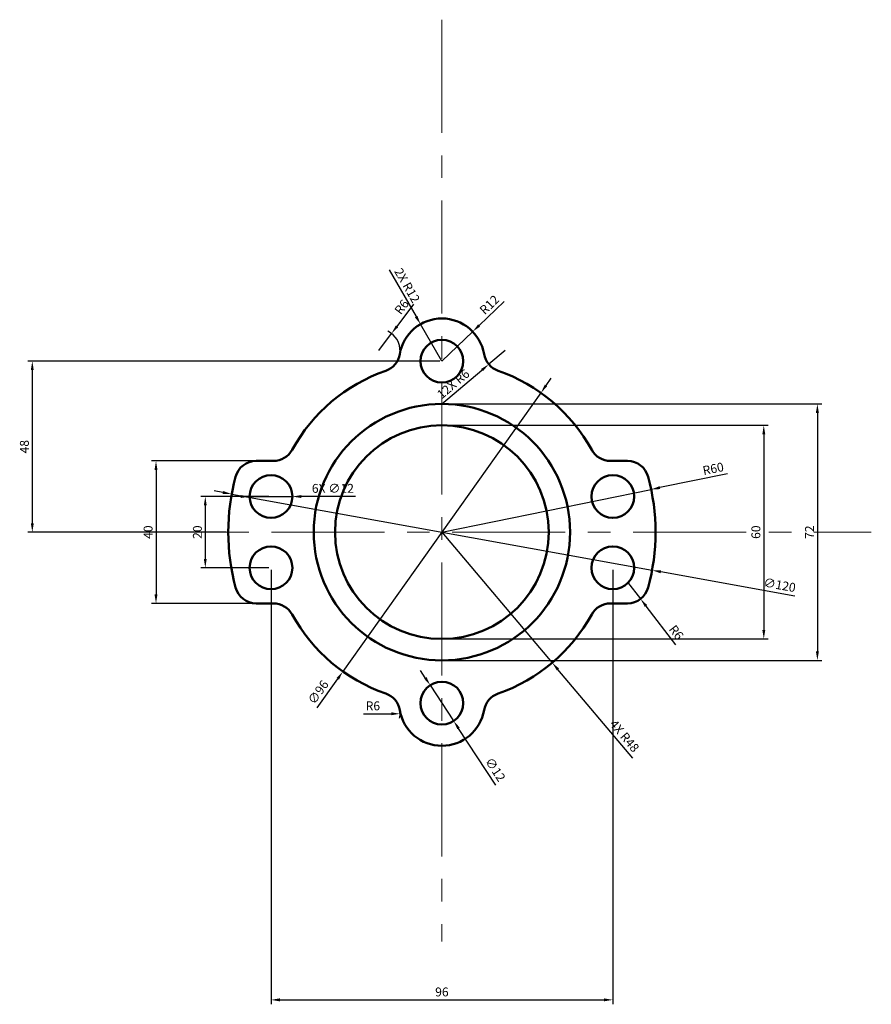
# Model space of a CAD drawing. Units: millimetres. Extents: x 2281 to 2520, y 1488 to 1764.
import ezdxf

# ---------------------------------------------------------------- set-up
doc = ezdxf.new("R2010")
doc.units = ezdxf.units.MM
doc.linetypes.add('CENTER', pattern=[50.8, 31.75, -6.35, 6.35, -6.35])
for name, color, linetype, lineweight in [('M-CNTR', 4, 'CENTER', 18), ('M-DIMS', 2, 'Continuous', 25), ('M-OUTL', 7, 'Continuous', 50)]:
    doc.layers.add(name, color=color, linetype=linetype, lineweight=lineweight)
doc.styles.get("Standard").update_dxf_attribs({"font": 'arial.ttf'})
doc.dimstyles.new('ISO-25', dxfattribs={"dimtxt": 2.5, "dimasz": 2.5, "dimexe": 1.25, "dimexo": 0.625, "dimtad": 1, "dimtxsty": 'Standard', "dimcen": 2.5, "dimadec": 0, "dimazin": 0, "dimtfac": 1, "dimtmove": 0, "dimatfit": 3, "dimfxl": 1, "dimarcsym": 0})

# ---------------------------------------------------------------- blocks, each defined once
blk = doc.blocks.new('*D1')
at = {"layer": 'Defpoints', "color": 0, "transparency": 16777216}
for p in [(2385.57, 1676.16), (2381.96, 1671.37)]:
    blk.add_point(p, dxfattribs=at)
at = {"layer": 'M-DIMS', "color": 0, "lineweight": -2, "transparency": 16777216}
for p, q in [((2391.76, 1684.37), (2387.08, 1678.16)), ((2381.96, 1671.37), (2385.57, 1676.16))]:
    blk.add_line(p, q, dxfattribs=at)
blk.add_arc((2381.96, 1671.37), 6, 356.3742, 64.8962, dxfattribs=at)
at = {"layer": 'M-DIMS', "color": 0, "transparency": 16777216}
blk.add_solid([(2386.75, 1678.41), (2387.41, 1677.91), (2385.57, 1676.16)], dxfattribs=at)
at = {"layer": 'M-DIMS', "color": 0, "transparency": 16777216, "insert": (2388.66, 1683.41), "char_height": 2.5, "attachment_point": 5, "rotation": 52.9596}
blk.add_mtext('R6', dxfattribs=at)
blk = doc.blocks.new('*D2')
at = {"layer": 'Defpoints', "color": 0, "transparency": 16777216}
for p in [(2408.36, 1676.69), (2399.71, 1668.37)]:
    blk.add_point(p, dxfattribs=at)
at = {"layer": 'M-DIMS', "color": 0, "lineweight": -2, "transparency": 16777216}
for p, q in [((2417.15, 1685.14), (2410.16, 1678.42)), ((2399.71, 1668.37), (2408.36, 1676.69))]:
    blk.add_line(p, q, dxfattribs=at)
at = {"layer": 'M-DIMS', "color": 0, "transparency": 16777216}
blk.add_solid([(2409.87, 1678.72), (2410.45, 1678.12), (2408.36, 1676.69)], dxfattribs=at)
at = {"layer": 'M-DIMS', "color": 0, "transparency": 16777216, "insert": (2413.26, 1684), "char_height": 2.5, "attachment_point": 5, "rotation": 43.8587}
blk.add_mtext('R12', dxfattribs=at)
blk = doc.blocks.new('*D3')
at = {"layer": 'Defpoints', "color": 0, "transparency": 16777216}
for p in [(2458.49, 1632.37), (2399.71, 1620.37)]:
    blk.add_point(p, dxfattribs=at)
at = {"layer": 'M-DIMS', "color": 0, "lineweight": -2, "transparency": 16777216}
for p, q in [((2479.89, 1636.74), (2460.94, 1632.87)), ((2399.71, 1620.37), (2458.49, 1632.37))]:
    blk.add_line(p, q, dxfattribs=at)
at = {"layer": 'M-DIMS', "color": 0, "transparency": 16777216}
blk.add_solid([(2460.86, 1633.28), (2461.03, 1632.46), (2458.49, 1632.37)], dxfattribs=at)
at = {"layer": 'M-DIMS', "color": 0, "transparency": 16777216, "insert": (2475.97, 1637.88), "char_height": 2.5, "attachment_point": 5, "rotation": 11.5363}
blk.add_mtext('R60', dxfattribs=at)
blk = doc.blocks.new('*D4')
at = {"layer": 'Defpoints', "color": 0, "transparency": 16777216}
for p in [(2451.86, 1606.37), (2455.51, 1601.61)]:
    blk.add_point(p, dxfattribs=at)
at = {"layer": 'M-DIMS', "color": 0, "lineweight": -2, "transparency": 16777216}
for p, q in [((2451.86, 1606.37), (2455.51, 1601.61)), ((2465.39, 1588.76), (2457.04, 1599.63))]:
    blk.add_line(p, q, dxfattribs=at)
at = {"layer": 'M-DIMS', "color": 0, "transparency": 16777216}
blk.add_solid([(2457.37, 1599.89), (2456.71, 1599.38), (2455.51, 1601.61)], dxfattribs=at)
at = {"layer": 'M-DIMS', "color": 0, "transparency": 16777216, "insert": (2465.29, 1592.02), "char_height": 2.5, "attachment_point": 5, "rotation": 307.5279}
blk.add_mtext('R6', dxfattribs=at)
blk = doc.blocks.new('*D5')
at = {"layer": 'Defpoints', "color": 0, "transparency": 16777216}
for p in [(2396.41, 1577.39), (2403, 1567.36)]:
    blk.add_point(p, dxfattribs=at)
at = {"layer": 'M-DIMS', "color": 0, "lineweight": -2, "transparency": 16777216}
for p, q in [((2395.03, 1579.47), (2393.66, 1581.56)), ((2396.41, 1577.39), (2403, 1567.36)), ((2414.87, 1549.32), (2404.38, 1565.27))]:
    blk.add_line(p, q, dxfattribs=at)
at = {"layer": 'M-DIMS', "color": 0, "transparency": 16777216}
for points in [[(2395.38, 1579.7), (2394.69, 1579.25), (2396.41, 1577.39)], [(2404.72, 1565.5), (2404.03, 1565.04), (2403, 1567.36)]]:
    blk.add_solid(points, dxfattribs=at)
at = {"layer": 'M-DIMS', "color": 0, "transparency": 16777216, "insert": (2414.45, 1553.55), "char_height": 2.5, "attachment_point": 5, "rotation": 303.334}
blk.add_mtext('∅12', dxfattribs=at)
blk = doc.blocks.new('*D6')
at = {"layer": 'Defpoints', "color": 0, "transparency": 16777216}
for p in [(2381.96, 1569.37), (2387.96, 1569.37)]:
    blk.add_point(p, dxfattribs=at)
at = {"layer": 'M-DIMS', "color": 0, "lineweight": -2, "transparency": 16777216}
blk.add_line((2377.68, 1569.37), (2385.46, 1569.37), dxfattribs=at)
blk.add_arc((2381.96, 1569.37), 6, 348.0634, 3.6258, dxfattribs=at)
at = {"layer": 'M-DIMS', "color": 0, "transparency": 16777216}
blk.add_solid([(2385.46, 1569.79), (2385.46, 1568.96), (2387.96, 1569.37)], dxfattribs=at)
at = {"layer": 'M-DIMS', "color": 0, "transparency": 16777216, "insert": (2380.32, 1571.27), "char_height": 2.5, "attachment_point": 5}
blk.add_mtext('R6', dxfattribs=at)
blk = doc.blocks.new('*D7')
at = {"layer": 'Defpoints', "color": 0, "transparency": 16777216}
for p in [(2427.51, 1659.5), (2371.9, 1581.24)]:
    blk.add_point(p, dxfattribs=at)
at = {"layer": 'M-DIMS', "color": 0, "lineweight": -2, "transparency": 16777216}
for p, q in [((2428.95, 1661.54), (2430.4, 1663.58)), ((2427.51, 1659.5), (2371.9, 1581.24)), ((2364.64, 1571.01), (2370.46, 1579.21))]:
    blk.add_line(p, q, dxfattribs=at)
at = {"layer": 'M-DIMS', "color": 0, "transparency": 16777216}
for points in [[(2428.62, 1661.78), (2429.29, 1661.3), (2427.51, 1659.5)], [(2370.12, 1579.45), (2370.8, 1578.96), (2371.9, 1581.24)]]:
    blk.add_solid(points, dxfattribs=at)
at = {"layer": 'M-DIMS', "color": 0, "transparency": 16777216, "insert": (2365.22, 1575.23), "char_height": 2.5, "attachment_point": 5, "rotation": 54.6066}
blk.add_mtext('∅96', dxfattribs=at)
blk = doc.blocks.new('*D8')
at = {"layer": 'Defpoints', "color": 0, "transparency": 16777216}
for p in [(2351.71, 1630.37), (2333.25, 1610.37), (2351.71, 1610.37)]:
    blk.add_point(p, dxfattribs=at)
at = {"layer": 'M-DIMS', "color": 0, "lineweight": -2, "transparency": 16777216}
for p, q in [((2351.08, 1630.37), (2332, 1630.37)), ((2333.25, 1627.87), (2333.25, 1612.87)), ((2351.08, 1610.37), (2332, 1610.37))]:
    blk.add_line(p, q, dxfattribs=at)
at = {"layer": 'M-DIMS', "color": 0, "transparency": 16777216}
for points in [[(2332.83, 1627.87), (2333.66, 1627.87), (2333.25, 1630.37)], [(2332.83, 1612.87), (2333.66, 1612.87), (2333.25, 1610.37)]]:
    blk.add_solid(points, dxfattribs=at)
at = {"layer": 'M-DIMS', "color": 0, "transparency": 16777216, "insert": (2331.35, 1620.37), "char_height": 2.5, "attachment_point": 5, "rotation": 90}
blk.add_mtext('20', dxfattribs=at)
blk = doc.blocks.new('*D9')
at = {"layer": 'Defpoints', "color": 0, "transparency": 16777216}
for p in [(2352.38, 1640.37), (2319.41, 1600.37), (2352.38, 1600.37)]:
    blk.add_point(p, dxfattribs=at)
at = {"layer": 'M-DIMS', "color": 0, "lineweight": -2, "transparency": 16777216}
for p, q in [((2351.75, 1640.37), (2318.16, 1640.37)), ((2319.41, 1637.87), (2319.41, 1602.87)), ((2351.75, 1600.37), (2318.16, 1600.37))]:
    blk.add_line(p, q, dxfattribs=at)
at = {"layer": 'M-DIMS', "color": 0, "transparency": 16777216}
for points in [[(2318.99, 1637.87), (2319.82, 1637.87), (2319.41, 1640.37)], [(2318.99, 1602.87), (2319.82, 1602.87), (2319.41, 1600.37)]]:
    blk.add_solid(points, dxfattribs=at)
at = {"layer": 'M-DIMS', "color": 0, "transparency": 16777216, "insert": (2317.51, 1620.37), "char_height": 2.5, "attachment_point": 5, "rotation": 90}
blk.add_mtext('40', dxfattribs=at)
blk = doc.blocks.new('*D10')
at = {"layer": 'Defpoints', "color": 0, "transparency": 16777216}
for p in [(2399.71, 1650.37), (2399.71, 1590.37), (2490.12, 1590.37)]:
    blk.add_point(p, dxfattribs=at)
at = {"layer": 'M-DIMS', "color": 0, "lineweight": -2, "transparency": 16777216}
for p, q in [((2400.33, 1650.37), (2491.37, 1650.37)), ((2490.12, 1647.87), (2490.12, 1592.87)), ((2400.33, 1590.37), (2491.37, 1590.37))]:
    blk.add_line(p, q, dxfattribs=at)
at = {"layer": 'M-DIMS', "color": 0, "transparency": 16777216}
for points in [[(2489.71, 1647.87), (2490.54, 1647.87), (2490.12, 1650.37)], [(2489.71, 1592.87), (2490.54, 1592.87), (2490.12, 1590.37)]]:
    blk.add_solid(points, dxfattribs=at)
at = {"layer": 'M-DIMS', "color": 0, "transparency": 16777216, "insert": (2488.22, 1620.37), "char_height": 2.5, "attachment_point": 5, "rotation": 90}
blk.add_mtext('60', dxfattribs=at)
blk = doc.blocks.new('*D11')
at = {"layer": 'Defpoints', "color": 0, "transparency": 16777216}
for p in [(2399.71, 1656.37), (2399.71, 1584.37), (2505.17, 1584.37)]:
    blk.add_point(p, dxfattribs=at)
at = {"layer": 'M-DIMS', "color": 0, "lineweight": -2, "transparency": 16777216}
for p, q in [((2400.33, 1656.37), (2506.42, 1656.37)), ((2505.17, 1653.87), (2505.17, 1586.87)), ((2400.33, 1584.37), (2506.42, 1584.37))]:
    blk.add_line(p, q, dxfattribs=at)
at = {"layer": 'M-DIMS', "color": 0, "transparency": 16777216}
for points in [[(2504.75, 1653.87), (2505.59, 1653.87), (2505.17, 1656.37)], [(2504.75, 1586.87), (2505.59, 1586.87), (2505.17, 1584.37)]]:
    blk.add_solid(points, dxfattribs=at)
at = {"layer": 'M-DIMS', "color": 0, "transparency": 16777216, "insert": (2503.29, 1620.37), "char_height": 2.5, "attachment_point": 5, "rotation": 90}
blk.add_mtext('72', dxfattribs=at)
blk = doc.blocks.new('BOLT-HOLE-D12')
blk.add_circle((6, 6), 6)
blk = doc.blocks.new('*D13')
at = {"layer": 'Defpoints', "color": 0, "transparency": 16777216}
for p in [(2351.71, 1610.37), (2447.71, 1610.37), (2447.71, 1489.03)]:
    blk.add_point(p, dxfattribs=at)
at = {"layer": 'M-DIMS', "color": 0, "lineweight": -2, "transparency": 16777216}
for p, q in [((2351.71, 1609.75), (2351.71, 1487.78)), ((2447.71, 1609.75), (2447.71, 1487.78)), ((2354.21, 1489.03), (2445.21, 1489.03))]:
    blk.add_line(p, q, dxfattribs=at)
at = {"layer": 'M-DIMS', "color": 0, "transparency": 16777216}
for points in [[(2354.21, 1489.45), (2354.21, 1488.61), (2351.71, 1489.03)], [(2445.21, 1489.45), (2445.21, 1488.61), (2447.71, 1489.03)]]:
    blk.add_solid(points, dxfattribs=at)
at = {"layer": 'M-DIMS', "color": 0, "transparency": 16777216, "insert": (2399.71, 1490.93), "char_height": 2.5, "attachment_point": 5}
blk.add_mtext('96', dxfattribs=at)
blk = doc.blocks.new('*D14')
at = {"layer": 'Defpoints', "color": 0, "transparency": 16777216}
for p in [(2399.71, 1668.37), (2284.66, 1620.37), (2339.71, 1620.37)]:
    blk.add_point(p, dxfattribs=at)
at = {"layer": 'M-DIMS', "color": 0, "lineweight": -2, "transparency": 16777216}
for p, q in [((2399.08, 1668.37), (2283.41, 1668.37)), ((2284.66, 1665.87), (2284.66, 1622.87)), ((2339.08, 1620.37), (2283.41, 1620.37))]:
    blk.add_line(p, q, dxfattribs=at)
at = {"layer": 'M-DIMS', "color": 0, "transparency": 16777216}
for points in [[(2284.24, 1665.87), (2285.07, 1665.87), (2284.66, 1668.37)], [(2284.24, 1622.87), (2285.07, 1622.87), (2284.66, 1620.37)]]:
    blk.add_solid(points, dxfattribs=at)
at = {"layer": 'M-DIMS', "color": 0, "transparency": 16777216, "insert": (2282.76, 1644.37), "char_height": 2.5, "attachment_point": 5, "rotation": 90}
blk.add_mtext('48', dxfattribs=at)
blk = doc.blocks.new('*D15')
at = {"layer": 'Defpoints', "color": 0, "transparency": 16777216}
for p in [(2340.67, 1631.06), (2458.75, 1609.69)]:
    blk.add_point(p, dxfattribs=at)
at = {"layer": 'M-DIMS', "color": 0, "lineweight": -2, "transparency": 16777216}
for p, q in [((2338.21, 1631.51), (2335.75, 1631.95)), ((2340.67, 1631.06), (2458.75, 1609.69)), ((2498.84, 1602.43), (2461.21, 1609.24))]:
    blk.add_line(p, q, dxfattribs=at)
at = {"layer": 'M-DIMS', "color": 0, "transparency": 16777216}
for points in [[(2338.28, 1631.92), (2338.13, 1631.1), (2340.67, 1631.06)], [(2461.28, 1609.65), (2461.13, 1608.83), (2458.75, 1609.69)]]:
    blk.add_solid(points, dxfattribs=at)
at = {"layer": 'M-DIMS', "color": 0, "transparency": 16777216, "insert": (2494.52, 1605.21), "char_height": 2.5, "attachment_point": 5, "rotation": 349.7398}
blk.add_mtext('∅120', dxfattribs=at)
blk = doc.blocks.new('*D16')
at = {"layer": 'Defpoints', "color": 0, "transparency": 16777216}
for p in [(2399.71, 1620.37), (2430.69, 1583.71)]:
    blk.add_point(p, dxfattribs=at)
at = {"layer": 'M-DIMS', "color": 0, "lineweight": -2, "transparency": 16777216}
for p, q in [((2399.71, 1620.37), (2430.69, 1583.71)), ((2453.38, 1556.87), (2432.3, 1581.8))]:
    blk.add_line(p, q, dxfattribs=at)
at = {"layer": 'M-DIMS', "color": 0, "transparency": 16777216}
blk.add_solid([(2432.62, 1582.07), (2431.99, 1581.53), (2430.69, 1583.71)], dxfattribs=at)
at = {"layer": 'M-DIMS', "color": 0, "transparency": 16777216, "insert": (2450.73, 1562.94), "char_height": 2.5, "attachment_point": 5, "rotation": 310.2035}
blk.add_mtext('4X R48', dxfattribs=at)
blk = doc.blocks.new('*D17')
at = {"layer": 'Defpoints', "color": 0, "transparency": 16777216}
for p in [(2393.71, 1678.77), (2399.71, 1668.37)]:
    blk.add_point(p, dxfattribs=at)
at = {"layer": 'M-DIMS', "color": 0, "lineweight": -2, "transparency": 16777216}
for p, q in [((2384.9, 1694.02), (2392.46, 1680.93)), ((2399.71, 1668.37), (2393.71, 1678.77))]:
    blk.add_line(p, q, dxfattribs=at)
at = {"layer": 'M-DIMS', "color": 0, "transparency": 16777216}
blk.add_solid([(2392.82, 1681.14), (2392.09, 1680.72), (2393.71, 1678.77)], dxfattribs=at)
at = {"layer": 'M-DIMS', "color": 0, "transparency": 16777216, "insert": (2389.68, 1689.5), "char_height": 2.5, "attachment_point": 5, "rotation": 300.0007}
blk.add_mtext('2X R12', dxfattribs=at)
blk = doc.blocks.new('*D18')
at = {"layer": 'Defpoints', "color": 0, "transparency": 16777216}
for p in [(2417.45, 1671.37), (2412.87, 1667.5)]:
    blk.add_point(p, dxfattribs=at)
at = {"layer": 'M-DIMS', "color": 0, "lineweight": -2, "transparency": 16777216}
for p, q in [((2417.45, 1671.37), (2412.87, 1667.5)), ((2399.62, 1656.29), (2410.96, 1665.89))]:
    blk.add_line(p, q, dxfattribs=at)
at = {"layer": 'M-DIMS', "color": 0, "transparency": 16777216}
blk.add_solid([(2410.69, 1666.2), (2411.23, 1665.57), (2412.87, 1667.5)], dxfattribs=at)
at = {"layer": 'M-DIMS', "color": 0, "transparency": 16777216, "insert": (2403.11, 1661.74), "char_height": 2.5, "attachment_point": 5, "rotation": 40.208}
blk.add_mtext('12X R6', dxfattribs=at)
blk = doc.blocks.new('*D19')
at = {"layer": 'Defpoints', "color": 0, "transparency": 16777216}
for p in [(2345.71, 1630.37), (2357.71, 1630.37)]:
    blk.add_point(p, dxfattribs=at)
at = {"layer": 'M-DIMS', "color": 0, "lineweight": -2, "transparency": 16777216}
for p, q in [((2343.21, 1630.37), (2340.71, 1630.37)), ((2345.71, 1630.37), (2357.71, 1630.37)), ((2375.48, 1630.37), (2360.21, 1630.37))]:
    blk.add_line(p, q, dxfattribs=at)
at = {"layer": 'M-DIMS', "color": 0, "transparency": 16777216}
for points in [[(2343.21, 1630.79), (2343.21, 1629.96), (2345.71, 1630.37)], [(2360.21, 1630.79), (2360.21, 1629.96), (2357.71, 1630.37)]]:
    blk.add_solid(points, dxfattribs=at)
at = {"layer": 'M-DIMS', "color": 0, "transparency": 16777216, "insert": (2369.09, 1632.34), "char_height": 2.5, "attachment_point": 5, "rotation": 359.9975}
blk.add_mtext('6X ∅12', dxfattribs=at)

msp = doc.modelspace()

# ---------------------------------------------------------------- linework, layer by layer
at = {"layer": 'M-CNTR'}
for p, q in [((2399.706, 1764.281), (2399.706, 1505.382)), ((2301.008, 1620.373), (2520.32, 1620.373))]:
    msp.add_line(p, q, dxfattribs=at)
at = {"layer": 'M-OUTL'}
for p, q in [((2347.552, 1640.373), (2352.377, 1640.373)), ((2451.859, 1640.373), (2447.034, 1640.373)), ((2347.552, 1600.373), (2352.377, 1600.373)), ((2451.859, 1600.373), (2447.034, 1600.373))]:
    msp.add_line(p, q, dxfattribs=at)
for radius in [36, 30]:
    msp.add_circle((2399.706, 1620.373), radius, dxfattribs=at)
for centre, radius, start, end in [((2399.706, 1668.373), 12, 9.59407, 170.40593), ((2381.958, 1671.373), 6, 289.18814, 350.40593), ((2417.454, 1671.373), 6, 189.59407, 250.81186), ((2399.706, 1620.373), 48, 109.18814, 151.2178), ((2399.706, 1620.373), 48, 28.7822, 70.81186), ((2352.377, 1646.373), 6, 270, 331.2178), ((2447.034, 1646.373), 6, 208.7822, 270), ((2347.552, 1634.373), 6, 90, 164.97389), ((2451.859, 1634.373), 6, 15.02611, 90), ((2399.706, 1620.373), 60, 164.97389, 195.02611), ((2399.706, 1620.373), 60, 344.97389, 15.02611), ((2347.552, 1606.373), 6, 195.02611, 270), ((2451.859, 1606.373), 6, 270, 344.97389), ((2352.377, 1594.373), 6, 28.7822, 90), ((2447.034, 1594.373), 6, 90, 151.2178), ((2399.706, 1620.373), 48, 208.7822, 250.81186), ((2399.706, 1620.373), 48, 289.18814, 331.2178), ((2381.958, 1569.373), 6, 9.59407, 70.81186), ((2417.454, 1569.373), 6, 109.18814, 170.40593), ((2399.706, 1572.373), 12, 189.59407, 350.40593)]:
    msp.add_arc(centre, radius, start, end, dxfattribs=at)

# ---------------------------------------------------------------- block references
for p in [(2393.706, 1662.373), (2345.706, 1624.373), (2441.706, 1624.373), (2345.706, 1604.373), (2441.706, 1604.373), (2393.706, 1566.373)]:
    msp.add_blockref('BOLT-HOLE-D12', p, dxfattribs=at)

# ---------------------------------------------------------------- dimensions: what is measured, and where the dimension line sits
at = {"layer": 'M-DIMS'}
for center, mpoint, text, picture, middle in [((2399.706, 1668.373), (2393.706, 1678.765), '2X <>', '*D17', (2389.681, 1689.497)), ((2417.454, 1671.373), (2412.872, 1667.5), '12X <>', '*D18', (2403.107, 1661.735))]:
    dim = msp.add_radius_dim(center=center, mpoint=mpoint, text=text, dimstyle='ISO-25', override={"dimdec": 0, "dimlfac": 1, "dimrnd": 0, "dimzin": 0, "dimdsep": 46, "dimlunit": 2}, dxfattribs=at)
    dim.commit()
    dim.dimension.update_dxf_attribs({"geometry": picture, "text_midpoint": middle})
for center, mpoint, picture, middle in [((2399.706, 1668.373), (2408.358, 1676.688), '*D2', (2413.256, 1684.002)), ((2381.958, 1671.373), (2385.572, 1676.163), '*D1', (2388.656, 1683.406))]:
    dim = msp.add_radius_dim(center=center, mpoint=mpoint, dimstyle='ISO-25', override={"dimclrd": 0, "dimclre": 0, "dimclrt": 0}, dxfattribs=at)
    dim.commit()
    dim.dimension.update_dxf_attribs({"geometry": picture, "text_midpoint": middle})
for base, p1, p2, override, picture, middle in [((2284.658, 1620.373), (2399.706, 1668.373), (2339.706, 1620.373), {"dimdec": 0, "dimlfac": 1, "dimrnd": 0, "dimzin": 0, "dimdsep": 46, "dimlunit": 2}, '*D14', (2282.757, 1644.373)), ((2505.17, 1584.373), (2399.706, 1656.373), (2399.706, 1584.373), {"dimclrd": 0, "dimclre": 0, "dimclrt": 0}, '*D11', (2503.29, 1620.373)), ((2490.122, 1590.373), (2399.706, 1650.373), (2399.706, 1590.373), {"dimclrd": 0, "dimclre": 0, "dimclrt": 0}, '*D10', (2488.22, 1620.373)), ((2319.408, 1600.373), (2352.377, 1640.373), (2352.377, 1600.373), {"dimclrd": 0, "dimclre": 0, "dimclrt": 0}, '*D9', (2317.506, 1620.373)), ((2333.248, 1610.373), (2351.706, 1630.373), (2351.706, 1610.373), {"dimclrd": 0, "dimclre": 0, "dimclrt": 0}, '*D8', (2331.346, 1620.373))]:
    dim = msp.add_linear_dim(base=base, p1=p1, p2=p2, angle=90, dimstyle='ISO-25', override=override, dxfattribs=at)
    dim.commit()
    dim.dimension.update_dxf_attribs({"geometry": picture, "text_midpoint": middle})
dim = msp.add_diameter_dim_2p(p1=(2427.507, 1659.503), p2=(2371.905, 1581.244), dimstyle='ISO-25', override={"dimclrd": 0, "dimclre": 0, "dimclrt": 0}, dxfattribs=at)
dim.commit()
dim.dimension.update_dxf_attribs({"geometry": '*D7', "text_midpoint": (2365.216, 1575.233)})
for center, mpoint, picture, middle in [((2399.706, 1620.373), (2458.494, 1632.373), '*D3', (2476.354, 1636.018)), ((2451.859, 1606.373), (2455.514, 1601.615), '*D4', (2463.777, 1590.857)), ((2381.958, 1569.373), (2387.958, 1569.373), '*D6', (2380.318, 1569.373))]:
    dim = msp.add_radius_dim(center=center, mpoint=mpoint, dimstyle='ISO-25', override={"dimclrd": 0, "dimclre": 0, "dimclrt": 0}, dxfattribs=at)
    dim.commit()
    dim.dimension.update_dxf_attribs({"geometry": picture, "text_midpoint": middle, "dimtype": 164})
dim = msp.add_diameter_dim_2p(p1=(2345.706, 1630.374), p2=(2357.706, 1630.373), text='6X <>', dimstyle='ISO-25', override={"dimdec": 0, "dimlfac": 1, "dimrnd": 0, "dimzin": 0, "dimdsep": 46, "dimlunit": 2}, dxfattribs=at)
dim.commit()
dim.dimension.update_dxf_attribs({"geometry": '*D19', "text_midpoint": (2369.095, 1630.373)})
for p1, p2, override, picture, middle in [((2340.665, 1631.06), (2458.746, 1609.686), {"dimdec": 0, "dimlfac": 1, "dimrnd": 0, "dimzin": 0, "dimdsep": 46, "dimlunit": 2}, '*D15', (2494.171, 1603.274)), ((2396.409, 1577.386), (2403.003, 1567.36), {"dimclrd": 0, "dimclre": 0, "dimclrt": 0}, '*D5', (2412.802, 1552.462))]:
    dim = msp.add_diameter_dim_2p(p1=p1, p2=p2, dimstyle='ISO-25', override=override, dxfattribs=at)
    dim.commit()
    dim.dimension.update_dxf_attribs({"geometry": picture, "text_midpoint": middle, "dimtype": 163})
dim = msp.add_radius_dim(center=(2399.706, 1620.373), mpoint=(2430.69, 1583.713), text='4X <>', dimstyle='ISO-25', override={"dimdec": 0, "dimlfac": 1, "dimrnd": 0, "dimzin": 0, "dimdsep": 46, "dimlunit": 2}, dxfattribs=at)
dim.commit()
dim.dimension.update_dxf_attribs({"geometry": '*D16', "text_midpoint": (2449.281, 1561.717), "dimtype": 164})
dim = msp.add_linear_dim(base=(2447.706, 1489.032), p1=(2351.706, 1610.373), p2=(2447.706, 1610.373), dimstyle='ISO-25', override={"dimdec": 0, "dimlfac": 1, "dimrnd": 0, "dimzin": 0, "dimdsep": 46, "dimlunit": 2}, dxfattribs=at)
dim.commit()
dim.dimension.update_dxf_attribs({"geometry": '*D13', "text_midpoint": (2399.706, 1490.933)})

doc.saveas('drawing.dxf')
